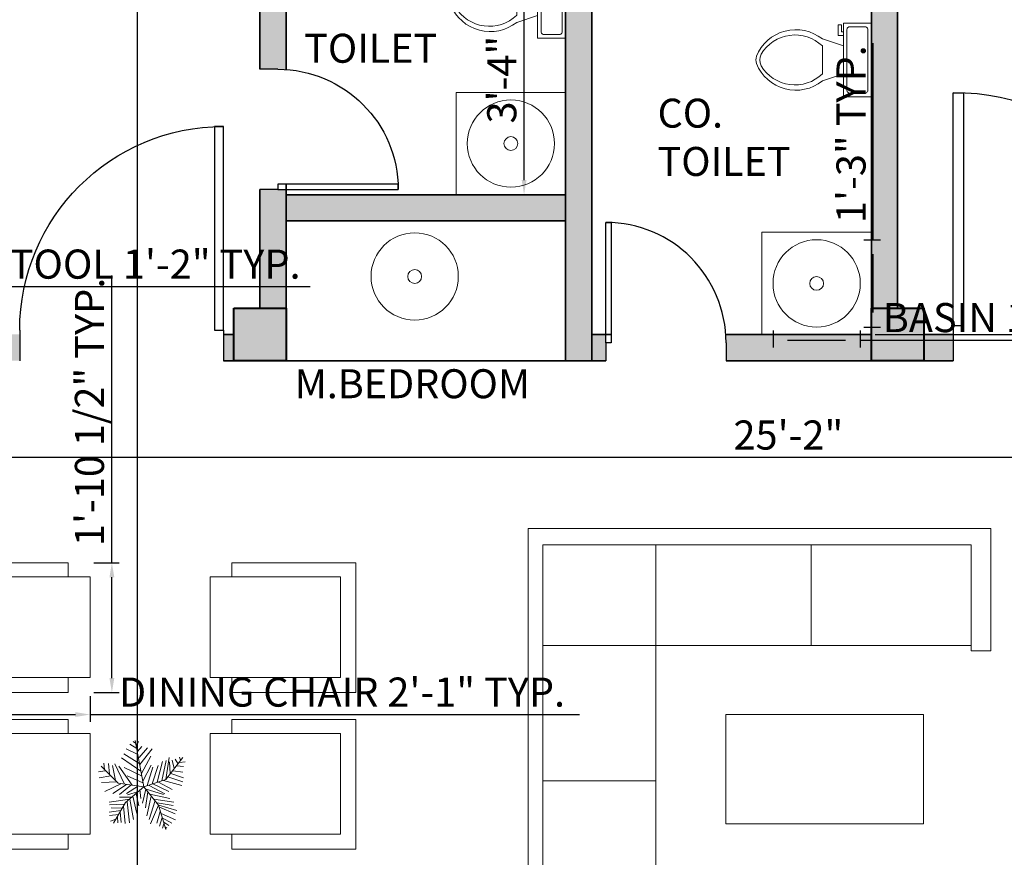
# Model space of a CAD drawing. Units: inches. Extents: x 1674 to 2231, y 1328 to 1959.
# Tile 4 of 6: x 1841 to 2010, y 1664 to 1807. Entities that reach past the tile are written whole.
import ezdxf

# ---------------------------------------------------------------- set-up
doc = ezdxf.new("R2010")
doc.units = ezdxf.units.IN
for name, color, linetype, lineweight in [('A-ANNO-DIMS', 113, 'Continuous', 18), ('A-AREA-IDEN', 113, 'Continuous', 18), ('A-COLS-PATT', 10, 'Continuous', 13), ('A-FLOR-FIXT', 211, 'Continuous', 18), ('A-WALL-PATT', 140, 'Continuous', 13), ('COLUMN', 10, 'Continuous', 40), ('DOOR', 54, 'Continuous', 25), ('FUR', 211, 'Continuous', 18), ('TREE', 102, 'Continuous', 13), ('WALL', 7, 'Continuous', 35)]:
    doc.layers.add(name, color=color, linetype=linetype, lineweight=lineweight)
doc.styles.get("Standard").update_dxf_attribs({"font": 'arial.ttf'})
doc.dimstyles.new('ISO-25', dxfattribs={"dimtxt": 5, "dimasz": 2.5, "dimexe": 1.25, "dimexo": 0.625, "dimtad": 1, "dimdec": 0, "dimlunit": 4, "dimtxsty": 'Standard', "dimcen": 2.5, "dimadec": 0, "dimazin": 0, "dimtfac": 1, "dimtdec": 0, "dimtmove": 0, "dimatfit": 3, "dimfxl": 1, "dimarcsym": 0})

# ---------------------------------------------------------------- blocks, each defined once
blk = doc.blocks.new('*U8')
for p, q in [((-8.737, 47.138), (-17.069, 52.711)), ((-10.186, 53.64), (-13.084, 55.962)), ((0, 0), (-10.5, 57)), ((-9.099, 51.782), (-6.563, 55.962)), ((-7.65, 43.423), (-2.578, 49.46)), ((-5.114, 28.097), (-24.676, 40.636)), ((-7.288, 39.707), (-21.778, 46.673)), ((-5.839, 35.992), (4.667, 48.067)), ((-5.114, 27.632), (10.463, 46.673)), ((-2.941, 16.486), (8.652, 37.85)), ((44.153, 36.456), (45.239, 32.741)), ((-31.5, 4.5), (-52.5, 25.5)), ((-48.585, 21.131), (-49.309, 29.026)), ((-43.513, 28.561), (-42.427, 15.558)), ((-38.442, 26.239), (-34.819, 7.663)), ((-35.544, 28.097), (-24.314, 3.947)), ((-14.533, 2.09), (-30.834, 25.31)), ((-3.665, 19.273), (-27.574, 35.527)), ((-1.129, 6.734), (9.014, 26.704)), ((3.942, 1.625), (11.187, 24.381)), ((10.101, 3.483), (17.708, 26.239)), ((16.259, 5.805), (23.142, 31.348)), ((22.055, 7.198), (27.489, 32.277)), ((27, 9), (48, 36)), ((27.127, 9.056), (31.112, 35.992)), ((31.836, 30.883), (32.561, 16.486)), ((35.096, 32.741), (37.27, 22.524)), ((38.719, 34.134), (41.979, 28.561)), ((40.53, 25.775), (48.862, 24.846)), ((43.791, 29.954), (51.036, 30.883)), ((-47.498, 19.737), (-55.83, 18.344)), ((-40.615, 13.7), (-55.105, 10.913)), ((-24.314, 23.917), (-2.941, 13.7)), ((-20.691, 13.7), (-1.129, 4.876)), ((29.662, 12.307), (48.137, 6.269)), ((33.285, 16.486), (48.862, 10.913)), ((36.183, 19.737), (48.137, 17.88)), ((-33.37, 6.269), (-52.207, 5.34)), ((-28.299, 3.483), (-47.86, -5.805)), ((-21.416, 3.018), (-38.079, -8.128)), ((0, 0), (-31.5, 4.5)), ((-15.982, 2.09), (-30.11, -9.521)), ((0, 0), (-22.5, -19.5)), ((-6.563, 1.161), (-21.416, -8.128)), ((0, 0), (27, 9)), ((0, 0), (18, -22.5)), ((6.478, 1.625), (26.04, -8.592)), ((11.187, 3.483), (30.749, -5.805)), ((18.07, 5.805), (35.096, -3.483)), ((24.229, 7.663), (46.688, 1.625)), ((-6.563, -5.805), (-19.967, -9.985)), ((-13.446, -11.378), (-8.737, -32.741)), ((-9.461, -8.592), (-6.201, -23.453)), ((-4.752, -3.483), (-3.665, -14.629)), ((2.493, -3.019), (-1.491, -20.202)), ((1.769, -2.555), (24.229, -9.521)), ((5.029, -6.27), (2.131, -25.775)), ((9.014, -11.378), (3.58, -35.992)), ((7.565, -9.056), (32.198, -14.629)), ((-17.431, -15.094), (-42.789, -18.809)), ((-24.314, -21.596), (-42.427, -22.06)), ((-22.5, -19.5), (-37.5, -45)), ((-15.257, -12.772), (-30.11, -12.772)), ((-25.038, -23.918), (-22.865, -45.281)), ((-20.691, -18.345), (-17.793, -44.352)), ((-17.069, -15.094), (-12.721, -40.172)), ((14.085, -16.951), (6.478, -40.172)), ((18.07, -22.524), (8.289, -45.745)), ((12.274, -15.094), (36.907, -18.809)), ((16.259, -19.738), (36.183, -22.989)), ((18, -22.5), (27, -52.5)), ((18.433, -22.524), (40.53, -29.026)), ((-28.299, -29.026), (-42.789, -31.348)), ((-30.834, -34.135), (-42.427, -35.528)), ((-26.849, -26.24), (-40.253, -25.775)), ((-29.023, -30.884), (-27.936, -43.887)), ((20.244, -30.419), (15.897, -44.816)), ((19.157, -25.311), (38.719, -33.206)), ((21.331, -32.741), (39.081, -40.636)), ((-34.457, -39.708), (-40.978, -42.494)), ((-32.646, -36.921), (-31.921, -44.352)), ((22.78, -37.85), (19.519, -48.532)), ((22.78, -38.314), (34.372, -44.816)), ((24.591, -45.745), (23.142, -50.854)), ((24.591, -43.423), (30.749, -47.603)), ((26.764, -49.925), (28.213, -50.854))]:
    blk.add_line(p, q)
blk = doc.blocks.new('*U2')
for p, q in [((0, 0), (0, -6)), ((40, 0), (40, -6))]:
    blk.add_line(p, q)
blk.add_lwpolyline([(0, 0), (0, 40), (1.75, 40), (1.75, 0)], close=True)
blk.add_arc((0, 0), 40, 0, 90)
blk = doc.blocks.new('*U4')
for p, q in [((9.5, -6), (9.5, -2)), ((-8, -8.5), (-8, -8)), ((-7, -8), (-7, -9.5)), ((-4, -8), (-6, -14)), ((4, -8), (6, -14)), ((-10, -8.5), (-8, -8.5)), ((-10, -9.5), (-10, -8.5)), ((-7, -9.5), (-10, -9.5)), ((4, -14), (-4, -14))]:
    blk.add_line(p, q)
blk.add_lwpolyline([(10.5, -8), (10.5, 0), (-10.5, 0), (-10.5, -8)], close=True)
for points in [[(-9.5, -2), (-9.5, -6)], [(8.5, -1), (-8.5, -1)], [(-8.5, -7), (8.5, -7)]]:
    blk.add_lwpolyline(points)
for centre, radius, start, end in [((-8.62, -1.88), 0.884, 81.8699, 188.1301), ((8.62, -1.88), 0.884, 351.8699, 98.1301), ((-8.62, -6.12), 0.884, 171.8699, 278.1301), ((8.62, -6.12), 0.884, 261.8699, 8.1301), ((3.52, -21.58), 12.17, 141.4691, 247.9714), ((4.2, -21.82), 11.33, 136.3677, 238.9468), ((-3.52, -21.58), 12.17, 292.0284, 38.5307), ((-4.2, -21.82), 11.33, 301.053, 43.6321), ((0, -27.88), 4, 245.7318, 294.2682), ((0, -29), 4, 254.8605, 285.1395)]:
    blk.add_arc(centre, radius, start, end)
blk = doc.blocks.new('*D18')
at = {"layer": 'A-ANNO-DIMS', "color": 0, "lineweight": -2, "transparency": 16777216}
for p, q in [((1933.65, 1816.86), (1925.88, 1816.86)), ((1927.13, 1779.86), (1927.13, 1814.36)), ((1933.65, 1777.36), (1925.88, 1777.36))]:
    blk.add_line(p, q, dxfattribs=at)
at = {"layer": 'A-ANNO-DIMS', "color": 0, "lineweight": 100, "transparency": 16777216}
for points in [[(1926.72, 1814.36), (1927.55, 1814.36), (1927.13, 1816.86)], [(1926.72, 1779.86), (1927.55, 1779.86), (1927.13, 1777.36)]]:
    blk.add_solid(points, dxfattribs=at)
at = {"layer": 'Defpoints', "color": 0, "lineweight": 100, "transparency": 16777216}
for p in [(1927.13, 1816.86), (1934.27, 1816.86), (1934.27, 1777.36)]:
    blk.add_point(p, dxfattribs=at)
at = {"layer": 'A-ANNO-DIMS', "color": 0, "transparency": 16777216, "insert": (1923.95, 1797.11), "char_height": 5, "attachment_point": 5, "rotation": 90}
blk.add_mtext('3\'-4"', dxfattribs=at)
blk = doc.blocks.new('*D33')
at = {"layer": 'A-ANNO-DIMS', "color": 0, "lineweight": -2, "transparency": 16777216}
for p, q in [((1821.77, 1748.23), (1821.77, 1731.03)), ((2123.27, 1748.18), (2123.27, 1731.03)), ((1824.27, 1732.28), (2120.77, 1732.28))]:
    blk.add_line(p, q, dxfattribs=at)
at = {"layer": 'A-ANNO-DIMS', "color": 0, "lineweight": 100, "transparency": 16777216}
for points in [[(1824.27, 1732.69), (1824.27, 1731.86), (1821.77, 1732.28)], [(2120.77, 1732.69), (2120.77, 1731.86), (2123.27, 1732.28)]]:
    blk.add_solid(points, dxfattribs=at)
at = {"layer": 'Defpoints', "color": 0, "lineweight": 100, "transparency": 16777216}
for p in [(1821.77, 1748.86), (2123.27, 1748.81), (2123.27, 1732.28)]:
    blk.add_point(p, dxfattribs=at)
at = {"layer": 'A-ANNO-DIMS', "color": 0, "transparency": 16777216, "insert": (1972.52, 1735.45), "char_height": 5, "attachment_point": 5}
blk.add_mtext('25\'-2"', dxfattribs=at)
blk = doc.blocks.new('CHAIR-DINING')
for p, q in [((21.28, 22.31), (0, 22.31)), ((0, 22.31), (0, 0)), ((21.28, 19.89), (21.28, 22.31)), ((21.28, 0), (21.28, 2.58)), ((0, 0), (21.28, 0))]:
    blk.add_line(p, q)
blk.add_lwpolyline([(25.04, 19.89), (2.65, 19.89), (2.65, 2.58), (25.04, 2.58)], close=True)
blk = doc.blocks.new('BASIN-ROUND')
for radius in [7.49, 1.19]:
    blk.add_circle((7.49, 7.49), radius)
blk = doc.blocks.new('*D40')
at = {"layer": 'A-ANNO-DIMS', "color": 0, "lineweight": -2, "transparency": 16777216}
for p, q in [((1827.55, 1691.24), (1827.55, 1686.86)), ((1852.59, 1691.24), (1852.59, 1686.86)), ((1830.05, 1688.11), (1850.09, 1688.11)), ((1852.59, 1688.11), (1936.63, 1688.11))]:
    blk.add_line(p, q, dxfattribs=at)
at = {"layer": 'A-ANNO-DIMS', "color": 0, "lineweight": 100, "transparency": 16777216}
for points in [[(1830.05, 1688.53), (1830.05, 1687.7), (1827.55, 1688.11)], [(1850.09, 1688.53), (1850.09, 1687.7), (1852.59, 1688.11)]]:
    blk.add_solid(points, dxfattribs=at)
at = {"layer": 'Defpoints', "color": 0, "lineweight": 100, "transparency": 16777216}
for p in [(1827.55, 1691.87), (1852.59, 1691.87), (1852.59, 1688.11)]:
    blk.add_point(p, dxfattribs=at)
at = {"layer": 'A-ANNO-DIMS', "color": 0, "transparency": 16777216, "insert": (1895.86, 1691.32), "char_height": 5, "attachment_point": 5}
blk.add_mtext('DINING CHAIR 2\'-1" TYP.', dxfattribs=at)
blk = doc.blocks.new('*D41')
at = {"layer": 'A-ANNO-DIMS', "color": 0, "lineweight": -2, "transparency": 16777216}
for p, q in [((1856.35, 1714.18), (1856.35, 1763.47)), ((1853.22, 1714.18), (1857.6, 1714.18)), ((1856.35, 1694.37), (1856.35, 1711.68)), ((1853.22, 1691.87), (1857.6, 1691.87))]:
    blk.add_line(p, q, dxfattribs=at)
at = {"layer": 'A-ANNO-DIMS', "color": 0, "lineweight": 100, "transparency": 16777216}
for points in [[(1855.93, 1711.68), (1856.76, 1711.68), (1856.35, 1714.18)], [(1855.93, 1694.37), (1856.76, 1694.37), (1856.35, 1691.87)]]:
    blk.add_solid(points, dxfattribs=at)
at = {"layer": 'Defpoints', "color": 0, "lineweight": 100, "transparency": 16777216}
for p in [(1852.59, 1714.18), (1856.35, 1714.18), (1852.59, 1691.87)]:
    blk.add_point(p, dxfattribs=at)
at = {"layer": 'A-ANNO-DIMS', "color": 0, "transparency": 16777216, "insert": (1853.14, 1740.07), "char_height": 5, "attachment_point": 5, "rotation": 90}
blk.add_mtext('1\'-10 1/2" TYP.', dxfattribs=at)
blk = doc.blocks.new('*D42')
at = {"layer": 'A-ANNO-DIMS', "color": 0, "lineweight": -2, "transparency": 16777216}
for p, q in [((1969.88, 1754.02), (1969.88, 1751.15)), ((1984.85, 1754.02), (1984.85, 1751.15)), ((1972.38, 1752.4), (1982.35, 1752.4)), ((1984.85, 1752.4), (2041.76, 1752.4))]:
    blk.add_line(p, q, dxfattribs=at)
at = {"layer": 'A-ANNO-DIMS', "color": 0, "lineweight": 100, "transparency": 16777216}
for points in [[(1972.38, 1752.81), (1972.38, 1751.98), (1969.88, 1752.4)], [(1982.35, 1752.81), (1982.35, 1751.98), (1984.85, 1752.4)]]:
    blk.add_solid(points, dxfattribs=at)
at = {"layer": 'Defpoints', "color": 0, "lineweight": 100, "transparency": 16777216}
for p in [(1969.88, 1754.64), (1984.85, 1754.64), (1984.85, 1752.4)]:
    blk.add_point(p, dxfattribs=at)
at = {"layer": 'A-ANNO-DIMS', "color": 0, "transparency": 16777216, "insert": (2014.56, 1755.61), "char_height": 5, "attachment_point": 5}
blk.add_mtext('BASIN 1\'-3" TYP.', dxfattribs=at)
blk = doc.blocks.new('*D43')
at = {"layer": 'A-ANNO-DIMS', "color": 0, "lineweight": -2, "transparency": 16777216}
for p, q in [((1987.1, 1769.62), (1987.1, 1803.38)), ((1985.48, 1769.62), (1988.35, 1769.62)), ((1987.1, 1757.14), (1987.1, 1767.12)), ((1985.48, 1754.64), (1988.35, 1754.64))]:
    blk.add_line(p, q, dxfattribs=at)
at = {"layer": 'A-ANNO-DIMS', "color": 0, "lineweight": 100, "transparency": 16777216}
for points in [[(1986.68, 1767.12), (1987.52, 1767.12), (1987.1, 1769.62)], [(1986.68, 1757.14), (1987.52, 1757.14), (1987.1, 1754.64)]]:
    blk.add_solid(points, dxfattribs=at)
at = {"layer": 'Defpoints', "color": 0, "lineweight": 100, "transparency": 16777216}
for p in [(1984.85, 1769.62), (1987.1, 1769.62), (1984.85, 1754.64)]:
    blk.add_point(p, dxfattribs=at)
at = {"layer": 'A-ANNO-DIMS', "color": 0, "transparency": 16777216, "insert": (1983.92, 1787.75), "char_height": 5, "attachment_point": 5, "rotation": 90}
blk.add_mtext('1\'-3" TYP.', dxfattribs=at)
blk = doc.blocks.new('*D48')
at = {"layer": 'A-ANNO-DIMS', "color": 0, "lineweight": -2, "transparency": 16777216}
for p, q in [((1816.72, 1763.03), (1816.72, 1760.33)), ((1830.58, 1763.03), (1830.58, 1760.33)), ((1819.22, 1761.58), (1828.08, 1761.58)), ((1830.58, 1761.58), (1890.4, 1761.58))]:
    blk.add_line(p, q, dxfattribs=at)
at = {"layer": 'A-ANNO-DIMS', "color": 0, "lineweight": 100, "transparency": 16777216}
for points in [[(1819.22, 1762), (1819.22, 1761.16), (1816.72, 1761.58)], [(1828.08, 1762), (1828.08, 1761.16), (1830.58, 1761.58)]]:
    blk.add_solid(points, dxfattribs=at)
at = {"layer": 'Defpoints', "color": 0, "lineweight": 100, "transparency": 16777216}
for p in [(1816.72, 1763.66), (1830.58, 1763.66), (1830.58, 1761.58)]:
    blk.add_point(p, dxfattribs=at)
at = {"layer": 'A-ANNO-DIMS', "color": 0, "transparency": 16777216, "insert": (1861.74, 1764.79), "char_height": 5, "attachment_point": 5}
blk.add_mtext('STOOL 1\'-2" TYP.', dxfattribs=at)
blk = doc.blocks.new('*D52')
at = {"layer": 'A-ANNO-DIMS', "color": 0, "lineweight": -2, "transparency": 16777216}
for p, q in [((1987.4, 1813.86), (2163.12, 1813.86)), ((2161.87, 1755.86), (2161.87, 1811.36)), ((1987.4, 1753.36), (2163.12, 1753.36))]:
    blk.add_line(p, q, dxfattribs=at)
at = {"layer": 'A-ANNO-DIMS', "color": 0, "lineweight": 100, "transparency": 16777216}
for points in [[(2161.45, 1811.36), (2162.29, 1811.36), (2161.87, 1813.86)], [(2161.45, 1755.86), (2162.29, 1755.86), (2161.87, 1753.36)]]:
    blk.add_solid(points, dxfattribs=at)
at = {"layer": 'Defpoints', "color": 0, "lineweight": 100, "transparency": 16777216}
for p in [(1986.77, 1813.86), (2161.87, 1813.86), (1986.77, 1753.36)]:
    blk.add_point(p, dxfattribs=at)
at = {"layer": 'A-ANNO-DIMS', "color": 0, "transparency": 16777216, "insert": (2158.66, 1783.61), "char_height": 5, "attachment_point": 5, "rotation": 90}
blk.add_mtext('5\'-0 1/2"', dxfattribs=at)
blk = doc.blocks.new('*D56')
at = {"layer": 'A-ANNO-DIMS', "color": 0, "lineweight": -2, "transparency": 16777216}
for p, q in [((1825.14, 1600.98), (1825.14, 1949.21)), ((1827.64, 1947.96), (1858.27, 1947.96)), ((1860.77, 1600.98), (1860.77, 1949.21))]:
    blk.add_line(p, q, dxfattribs=at)
at = {"layer": 'A-ANNO-DIMS', "color": 0, "lineweight": 100, "transparency": 16777216}
for points in [[(1827.64, 1948.37), (1827.64, 1947.54), (1825.14, 1947.96)], [(1858.27, 1948.37), (1858.27, 1947.54), (1860.77, 1947.96)]]:
    blk.add_solid(points, dxfattribs=at)
at = {"layer": 'Defpoints', "color": 0, "lineweight": 100, "transparency": 16777216}
for p in [(1860.77, 1947.96), (1825.14, 1600.36), (1860.77, 1600.36)]:
    blk.add_point(p, dxfattribs=at)
at = {"layer": 'A-ANNO-DIMS', "color": 0, "transparency": 16777216, "insert": (1842.96, 1951.17), "char_height": 5, "attachment_point": 5}
blk.add_mtext('2\'-11 1/2"', dxfattribs=at)

msp = doc.modelspace()

# ---------------------------------------------------------------- hatches: boundary and pattern name
at = {"layer": 'A-COLS-PATT'}
h = msp.add_hatch(color=256, dxfattribs=at)
h.dxf.hatch_style = 1
h.paths.add_polyline_path([(1745.27, 1918.36), (1736.27, 1918.36), (1736.27, 1909.36), (1745.27, 1909.36)])
h.paths.add_polyline_path([(1886.27, 1918.36), (1877.27, 1918.36), (1877.27, 1909.36), (1886.27, 1909.36)])
h.paths.add_polyline_path([(1995.77, 1918.36), (1986.77, 1918.36), (1986.77, 1909.36), (1995.77, 1909.36)])
h.paths.add_polyline_path([(2132.27, 1918.36), (2123.27, 1918.36), (2123.27, 1909.36), (2132.27, 1909.36)])
h.paths.add_polyline_path([(1745.27, 1757.86), (1736.27, 1757.86), (1736.27, 1748.86), (1745.27, 1748.86)])
h.paths.add_polyline_path([(1886.27, 1757.86), (1877.27, 1757.86), (1877.27, 1748.86), (1886.27, 1748.86)])
h.paths.add_polyline_path([(2132.27, 1757.81), (2123.27, 1757.81), (2123.27, 1748.81), (2132.27, 1748.81)])
h.paths.add_polyline_path([(1995.77, 1757.86), (1986.77, 1757.86), (1986.77, 1748.86), (1995.77, 1748.86)])
h.paths.add_polyline_path([(2132.27, 1625.36), (2123.27, 1625.36), (2123.27, 1616.36), (2132.27, 1616.36)])
h.paths.add_polyline_path([(1995.77, 1625.36), (1986.77, 1625.36), (1986.77, 1616.36), (1995.77, 1616.36)])
h.paths.add_polyline_path([(1869.77, 1604.86), (1860.77, 1604.86), (1860.77, 1595.86), (1869.77, 1595.86)])
h.paths.add_polyline_path([(1745.27, 1609.36), (1736.27, 1609.36), (1736.27, 1600.36), (1745.27, 1600.36)])
h.paths.add_polyline_path([(1745.27, 1504.36), (1736.27, 1504.36), (1736.27, 1495.36), (1745.27, 1495.36)])
h.paths.add_polyline_path([(1870.95, 1504.36), (1861.95, 1504.36), (1861.95, 1495.36), (1870.95, 1495.36)])
h.paths.add_polyline_path([(1995.77, 1504.36), (1986.77, 1504.36), (1986.77, 1495.36), (1995.77, 1495.36)])
h.paths.add_polyline_path([(1995.77, 1447.36), (1986.77, 1447.36), (1986.77, 1438.36), (1995.77, 1438.36)])
h.paths.add_polyline_path([(2132.27, 1447.36), (2123.27, 1447.36), (2123.27, 1438.36), (2132.27, 1438.36)])
at = {"layer": 'A-WALL-PATT'}
h = msp.add_hatch(color=256, dxfattribs=at)
h.dxf.hatch_style = 1
h.paths.add_polyline_path([(1877.27, 1918.36), (1745.27, 1918.36), (1745.27, 1909.36), (1877.27, 1909.36)])
h.paths.add_polyline_path([(1986.77, 1918.36), (1886.27, 1918.36), (1886.27, 1909.36), (1986.77, 1909.36)])
h.paths.add_polyline_path([(2123.27, 1918.36), (1995.77, 1918.36), (1995.77, 1909.36), (2123.27, 1909.36)])
h.paths.add_polyline_path([(1894.11, 1861.36), (1886.27, 1861.36), (1886.27, 1865.74), (1881.77, 1865.74), (1881.77, 1808), (1881.77, 1798.89), (1884.87, 1798.89, -0.017002), (1886.27, 1798.84), (1886.27, 1852.36), (1894.11, 1852.36)])
h.paths.add_polyline_path([(1952.87, 1861.36), (1919.24, 1861.36), (1919.24, 1852.36), (1952.87, 1852.36)])
h.paths.add_polyline_path([(1991.27, 1865.74), (1986.77, 1865.74), (1986.77, 1861.36), (1976.26, 1861.36), (1976.26, 1852.36), (1986.77, 1852.36), (1986.77, 1847.49), (1986.77, 1757.86), (1991.27, 1757.86), (1991.27, 1852.36)])
h.paths.add_polyline_path([(1986.77, 1816.36), (1938.77, 1816.36), (1938.77, 1813.86), (1986.77, 1813.86)])
h.paths.add_polyline_path([(1934.27, 1819.36), (1886.27, 1819.36), (1886.27, 1816.86), (1934.27, 1816.86)])
h.paths.add_polyline_path([(1938.77, 1852.36), (1934.27, 1852.36), (1934.27, 1753.36), (1934.27, 1748.86), (1938.77, 1748.86), (1938.77, 1753.36)])
h.paths.add_polyline_path([(1934.27, 1777.36), (1915.46, 1777.36), (1886.27, 1777.36), (1886.27, 1772.86), (1934.27, 1772.86)])
h.paths.add_polyline_path([(1986.77, 1753.36), (1967.96, 1753.36), (1961.77, 1753.36, -0.017002), (1961.81, 1751.95), (1961.81, 1748.86), (1986.77, 1748.86)])
h.paths.add_polyline_path([(2000.84, 1753.36), (1995.77, 1753.36), (1995.77, 1748.86), (2000.84, 1748.86)])
h.paths.add_polyline_path([(1941.17, 1751.95), (1941.17, 1753.36), (1938.77, 1753.36), (1938.77, 1748.86), (1941.17, 1748.86)])
h.paths.add_polyline_path([(1877.27, 1753.36), (1875.49, 1753.36), (1875.49, 1748.86), (1877.27, 1748.86)])
h.paths.add_polyline_path([(1745.27, 1909.36), (1736.27, 1909.36), (1736.27, 1757.86), (1745.27, 1757.86), (1745.27, 1773.01)])
h.paths.add_polyline_path([(1778.41, 1645.36), (1745.27, 1645.36), (1745.27, 1640.86), (1778.41, 1640.86)])
h.paths.add_polyline_path([(1821.77, 1645.36), (1821.77, 1668.45), (1817.27, 1668.45), (1817.27, 1645.36), (1817.27, 1640.86), (1821.77, 1640.86)])
h.paths.add_polyline_path([(1817.27, 1645.36), (1813.39, 1645.36), (1813.39, 1640.86), (1817.27, 1640.86)])
h.paths.add_polyline_path([(1821.77, 1640.86), (1817.27, 1640.86), (1817.27, 1604.86), (1817.27, 1600.36), (1821.77, 1600.36)])
h.paths.add_polyline_path([(1825.14, 1604.86), (1821.77, 1604.86), (1821.77, 1600.36), (1825.14, 1600.36)])
h.paths.add_polyline_path([(1781.27, 1604.86), (1745.27, 1604.86), (1745.27, 1600.36), (1781.27, 1600.36)])
h = msp.add_hatch(color=256, dxfattribs=at)
h.dxf.hatch_style = 1
h.paths.add_polyline_path([(2132.27, 1909.36), (2123.27, 1909.36), (2123.27, 1757.81), (2132.27, 1757.81)], flags=17)
h.paths.add_polyline_path([(2123.27, 1753.36), (2040.84, 1753.36), (2040.84, 1748.86), (2123.27, 1748.86)], flags=17)
h.paths.add_polyline_path([(1840.51, 1753.36), (1745.27, 1753.36), (1745.27, 1748.86), (1817.27, 1748.86), (1840.51, 1748.86)], flags=17)
h.paths.add_polyline_path([(1745.27, 1748.86), (1736.27, 1748.86), (1736.27, 1609.36), (1745.27, 1609.36), (1745.27, 1640.86)], flags=17)
h.paths.add_polyline_path([(1745.27, 1600.36), (1736.27, 1600.36), (1736.27, 1504.36), (1745.27, 1504.36)], flags=17)
h.paths.add_polyline_path([(1745.27, 1495.36), (1736.27, 1495.36), (1736.27, 1447.36), (1745.27, 1447.36)], flags=17)
h.paths.add_polyline_path([(1820.35, 1504.36), (1787.69, 1504.36), (1787.69, 1495.36), (1820.35, 1495.36)], flags=17)
h.paths.add_polyline_path([(1750.58, 1504.36), (1745.27, 1504.36), (1745.27, 1495.36), (1750.58, 1495.36)], flags=17)
h.paths.add_polyline_path([(1861.95, 1504.36), (1857.47, 1504.36), (1857.47, 1495.36), (1861.95, 1495.36)], flags=17)
h.paths.add_polyline_path([(1873.66, 1504.36), (1870.95, 1504.36), (1870.95, 1495.36), (1873.66, 1495.36)], flags=17)
h.paths.add_polyline_path([(1900.85, 1501.36), (1900.85, 1504.36), (1895.88, 1504.36), (1895.88, 1495.36), (1900.85, 1495.36)], flags=17)
h.paths.add_polyline_path([(1869.77, 1595.86), (1865.27, 1595.86), (1865.27, 1504.36), (1869.77, 1504.36)], flags=17)
h.paths.add_polyline_path([(1958.26, 1504.36), (1940.74, 1504.36, -0.01877), (1940.85, 1501.36), (1940.85, 1495.36), (1958.26, 1495.36)], flags=17)
h.paths.add_polyline_path([(1995.77, 1531.51), (1986.77, 1531.51), (1986.77, 1504.36), (1995.77, 1504.36)], flags=17)
h.paths.add_polyline_path([(1986.77, 1504.36), (1980.49, 1504.36), (1980.49, 1495.36), (1986.77, 1495.36)], flags=17)
h.paths.add_polyline_path([(1995.77, 1616.36), (1986.77, 1616.36), (1986.77, 1585.02), (1995.77, 1585.02)], flags=17)
h.paths.add_polyline_path([(2000.1, 1620.86), (1995.77, 1620.86), (1995.77, 1616.36), (2000.1, 1616.36)], flags=17)
h.paths.add_polyline_path([(2053.57, 1620.86), (2040.1, 1620.86), (2040.1, 1616.36), (2053.57, 1616.36)], flags=17)
h.paths.add_polyline_path([(2123.27, 1620.86), (2109.12, 1620.86), (2109.12, 1616.36), (2123.27, 1616.36)], flags=17)
h.paths.add_polyline_path([(2132.27, 1616.36), (2123.27, 1616.36), (2123.27, 1447.36), (2132.27, 1447.36)], flags=17)
h.paths.add_polyline_path([(1986.77, 1447.36), (1870.95, 1447.36), (1870.95, 1438.36), (1986.77, 1438.36)])
h.paths.add_polyline_path([(1861.95, 1447.36), (1745.27, 1447.36), (1745.27, 1438.36), (1861.95, 1438.36)])
h.paths.add_polyline_path([(2132.27, 1918.36), (1736.27, 1918.36), (1736.27, 1504.36), (1745.27, 1504.36), (1745.27, 1600.36), (1745.27, 1909.36), (2123.27, 1909.36), (2123.27, 1447.36), (2132.27, 1447.36)])
h = msp.add_hatch(color=256, dxfattribs=at)
h.dxf.hatch_style = 1
h.paths.add_polyline_path([(1886.27, 1777.36), (1886.27, 1778.24), (1884.87, 1778.24), (1881.77, 1778.24), (1881.77, 1757.86), (1886.27, 1757.86)], flags=17)
h.paths.add_polyline_path([(2132.27, 1918.36), (1736.27, 1918.36), (1736.27, 1757.86), (1745.27, 1757.86), (1745.27, 1773.01), (1745.27, 1909.36), (2123.27, 1909.36), (2123.27, 1757.81), (2132.27, 1757.81)])

# ---------------------------------------------------------------- linework, layer by layer
at = {"layer": 'A-FLOR-FIXT'}
for points in [[(1934.27, 1777.36), (1915.46, 1777.36), (1915.46, 1794.91), (1934.27, 1794.91)], [(1986.77, 1753.36), (1967.96, 1753.36), (1967.96, 1770.91), (1986.77, 1770.91)]]:
    msp.add_lwpolyline(points, close=True, dxfattribs=at)
at = {"layer": 'COLUMN'}
for points in [[(1877.27, 1757.86), (1886.27, 1757.86), (1886.27, 1748.86), (1877.27, 1748.86)], [(1986.77, 1757.86), (1995.77, 1757.86), (1995.77, 1748.86), (1986.77, 1748.86)]]:
    msp.add_lwpolyline(points, close=True, dxfattribs=at)
at = {"layer": 'FUR'}
for p, q in [((1927.85, 1652.61), (1927.85, 1720.04)), ((1927.85, 1720.04), (2007.29, 1720.04)), ((2007.29, 1720.04), (2007.29, 1699.07)), ((1976.41, 1717.22), (1976.41, 1699.95)), ((2003.89, 1699.95), (2003.89, 1699.07)), ((2007.29, 1699.07), (2003.89, 1699.07)), ((1930.34, 1676.73), (1949.77, 1676.73))]:
    msp.add_line(p, q, dxfattribs=at)
for points in [[(1930.34, 1717.22), (2003.89, 1717.22), (2003.89, 1699.95), (1930.34, 1699.95)], [(1930.34, 1717.22), (1949.77, 1717.22), (1949.77, 1655.93), (1930.34, 1655.93)], [(1961.75, 1688.1), (1995.7, 1688.1), (1995.7, 1669.36), (1961.75, 1669.36)]]:
    msp.add_lwpolyline(points, close=True, dxfattribs=at)
at = {"layer": 'WALL'}
for p, q in [((1881.77, 1909.36), (1881.77, 1798.89)), ((1886.27, 1852.36), (1886.27, 1798.84)), ((1934.27, 1852.36), (1934.27, 1753.36)), ((1938.77, 1852.36), (1938.77, 1753.36)), ((1986.77, 1852.36), (1986.77, 1753.36)), ((1991.27, 1852.36), (1991.27, 1757.86)), ((1934.27, 1819.36), (1934.27, 1753.36)), ((1886.27, 1779.15), (1886.27, 1753.36)), ((1881.77, 1778.24), (1881.77, 1757.86)), ((1886.27, 1753.36), (1886.27, 1777.36)), ((1886.27, 1777.36), (1934.27, 1777.36)), ((1886.27, 1772.86), (1934.27, 1772.86)), ((1877.27, 1753.36), (1875.49, 1753.36)), ((1934.27, 1753.36), (1934.27, 1748.86)), ((1938.77, 1753.36), (1942.07, 1753.36)), ((1938.77, 1753.36), (1938.77, 1748.86)), ((1961.77, 1753.36), (1986.77, 1753.36)), ((1995.77, 1753.36), (2000.84, 1753.36)), ((1886.27, 1748.86), (1875.49, 1748.86)), ((1886.27, 1748.86), (1934.27, 1748.86)), ((1934.27, 1748.86), (1941.17, 1748.86)), ((1961.81, 1748.86), (1986.77, 1748.86)), ((1986.77, 1748.86), (2000.84, 1748.86))]:
    msp.add_line(p, q, dxfattribs=at)

# ---------------------------------------------------------------- block references
at = {"layer": 'A-FLOR-FIXT', "xscale": 0.6007383453482145, "yscale": 0.6007383453482145, "zscale": 0.6007383453482145, "rotation": 270}
for p in [(1934.27, 1810.55), (1986.77, 1800.49)]:
    msp.add_blockref('*U4', p, dxfattribs=at)
at = {"layer": 'A-FLOR-FIXT'}
for p in [(1917.38, 1778.64), (1900.86, 1755.83), (1969.88, 1754.64)]:
    msp.add_blockref('BASIN-ROUND', p, dxfattribs=at)
at = {"layer": 'DOOR', "xscale": -0.5161744683548543, "yscale": 0.5161744683548543, "zscale": 0.5161744683548543, "rotation": 270}
msp.add_blockref('*U2', (1884.87, 1778.24), dxfattribs=at)
at = {"layer": 'DOOR'}
msp.add_blockref('*U2', (2000.84, 1754.86), dxfattribs=at)
for p, xscale, yscale, zscale in [((1875.49, 1754.1), -0.8744829560094038, 0.8744829560094038, 0.8744829560094038), ((1941.17, 1751.95), 0.5161744683548543, 0.5161744683548543, 0.5161744683548543)]:
    msp.add_blockref('*U2', p, dxfattribs=dict(at, xscale=xscale, yscale=yscale, zscale=zscale))
at = {"layer": 'FUR'}
for p in [(1827.55, 1691.87), (1827.55, 1664.98)]:
    msp.add_blockref('CHAIR-DINING', p, dxfattribs=at)
at = {"layer": 'FUR', "extrusion": (0, 0, -1), "zscale": -1}
for p in [(-1898.25, 1691.87), (-1898.25, 1664.98)]:
    msp.add_blockref('CHAIR-DINING', p, dxfattribs=at)
at = {"layer": 'TREE', "xscale": 0.1393019906957703, "yscale": 0.1393019906957703, "zscale": 0.1393019906957703}
msp.add_blockref('*U8', (1861.83, 1675.71), dxfattribs=at)

# ---------------------------------------------------------------- texts
at = {"layer": 'A-AREA-IDEN', "char_height": 4.973, "attachment_point": 1}
for s, insert in [('TOILET', (1889.38, 1804.98)), ('CO.\\PTOILET', (1950.06, 1793.84)), ('M.BEDROOM', (1887.75, 1747.39))]:
    msp.add_mtext_dynamic_manual_height_columns(s, width=89.7127, gutter_width=24.87, heights=[0], dxfattribs=dict(at, insert=insert))

# ---------------------------------------------------------------- dimensions: what is measured, and where the dimension line sits
at = {"layer": 'A-ANNO-DIMS'}
for base, p1, p2, override, picture, middle in [((1860.77, 1947.96), (1825.14, 1600.36), (1860.77, 1600.36), {"dimdec": 1, "dimlfac": 1, "dimrnd": 0, "dimzin": 1, "dimdsep": 46, "dimlunit": 4, "dimfrac": 2}, '*D56', (1842.96, 1951.17)), ((2123.27109151, 1732.2761534), (1821.77109151, 1748.85548105), (2123.27109151, 1748.80863988), {"dimclrd": 0, "dimclre": 0, "dimclrt": 0}, '*D33', (1972.52109151, 1735.45401834))]:
    dim = msp.add_linear_dim(base=base, p1=p1, p2=p2, dimstyle='ISO-25', override=override, dxfattribs=at)
    dim.commit()
    dim.dimension.update_dxf_attribs({"geometry": picture, "text_midpoint": middle})
for base, p1, p2, override, picture, middle in [((1927.13363559, 1816.85548105), (1934.27109151, 1777.35548105), (1934.27109151, 1816.85548105), {"dimclrd": 0, "dimclre": 0, "dimclrt": 0}, '*D18', (1923.95406533, 1797.10548105)), ((2161.87, 1813.86), (1986.77, 1753.36), (1986.77, 1813.86), {"dimdec": 1, "dimlfac": 1, "dimrnd": 0, "dimzin": 1, "dimdsep": 46, "dimlunit": 4, "dimfrac": 2}, '*D52', (2158.66, 1783.61))]:
    dim = msp.add_linear_dim(base=base, p1=p1, p2=p2, angle=90, dimstyle='ISO-25', override=override, dxfattribs=at)
    dim.commit()
    dim.dimension.update_dxf_attribs({"geometry": picture, "text_midpoint": middle})
for base, p1, p2, picture, middle in [((1987.1, 1769.62), (1984.85, 1754.64), (1984.85, 1769.62), '*D43', (1983.92, 1787.75)), ((1856.35, 1714.18), (1852.59, 1691.87), (1852.59, 1714.18), '*D41', (1853.14, 1740.07))]:
    dim = msp.add_linear_dim(base=base, p1=p1, p2=p2, angle=90, text='<> TYP.', dimstyle='ISO-25', override={"dimdec": 1, "dimlfac": 1, "dimrnd": 0, "dimzin": 1, "dimdsep": 46, "dimlunit": 4, "dimfrac": 2}, dxfattribs=at)
    dim.commit()
    dim.dimension.update_dxf_attribs({"geometry": picture, "text_midpoint": middle})
for base, p1, p2, text, picture, middle in [((1830.58, 1761.58), (1816.72, 1763.66), (1830.58, 1763.66), 'STOOL <> TYP.', '*D48', (1861.74, 1764.79)), ((1984.85, 1752.4), (1969.88, 1754.64), (1984.85, 1754.64), 'BASIN <> TYP.', '*D42', (2014.56, 1755.61)), ((1852.59, 1688.11), (1827.55, 1691.87), (1852.59, 1691.87), 'DINING CHAIR <> TYP.', '*D40', (1895.86, 1691.32))]:
    dim = msp.add_linear_dim(base=base, p1=p1, p2=p2, text=text, dimstyle='ISO-25', override={"dimdec": 1, "dimlfac": 1, "dimrnd": 0, "dimzin": 1, "dimdsep": 46, "dimlunit": 4, "dimfrac": 2}, dxfattribs=at)
    dim.commit()
    dim.dimension.update_dxf_attribs({"geometry": picture, "text_midpoint": middle})

doc.saveas('drawing.dxf')
